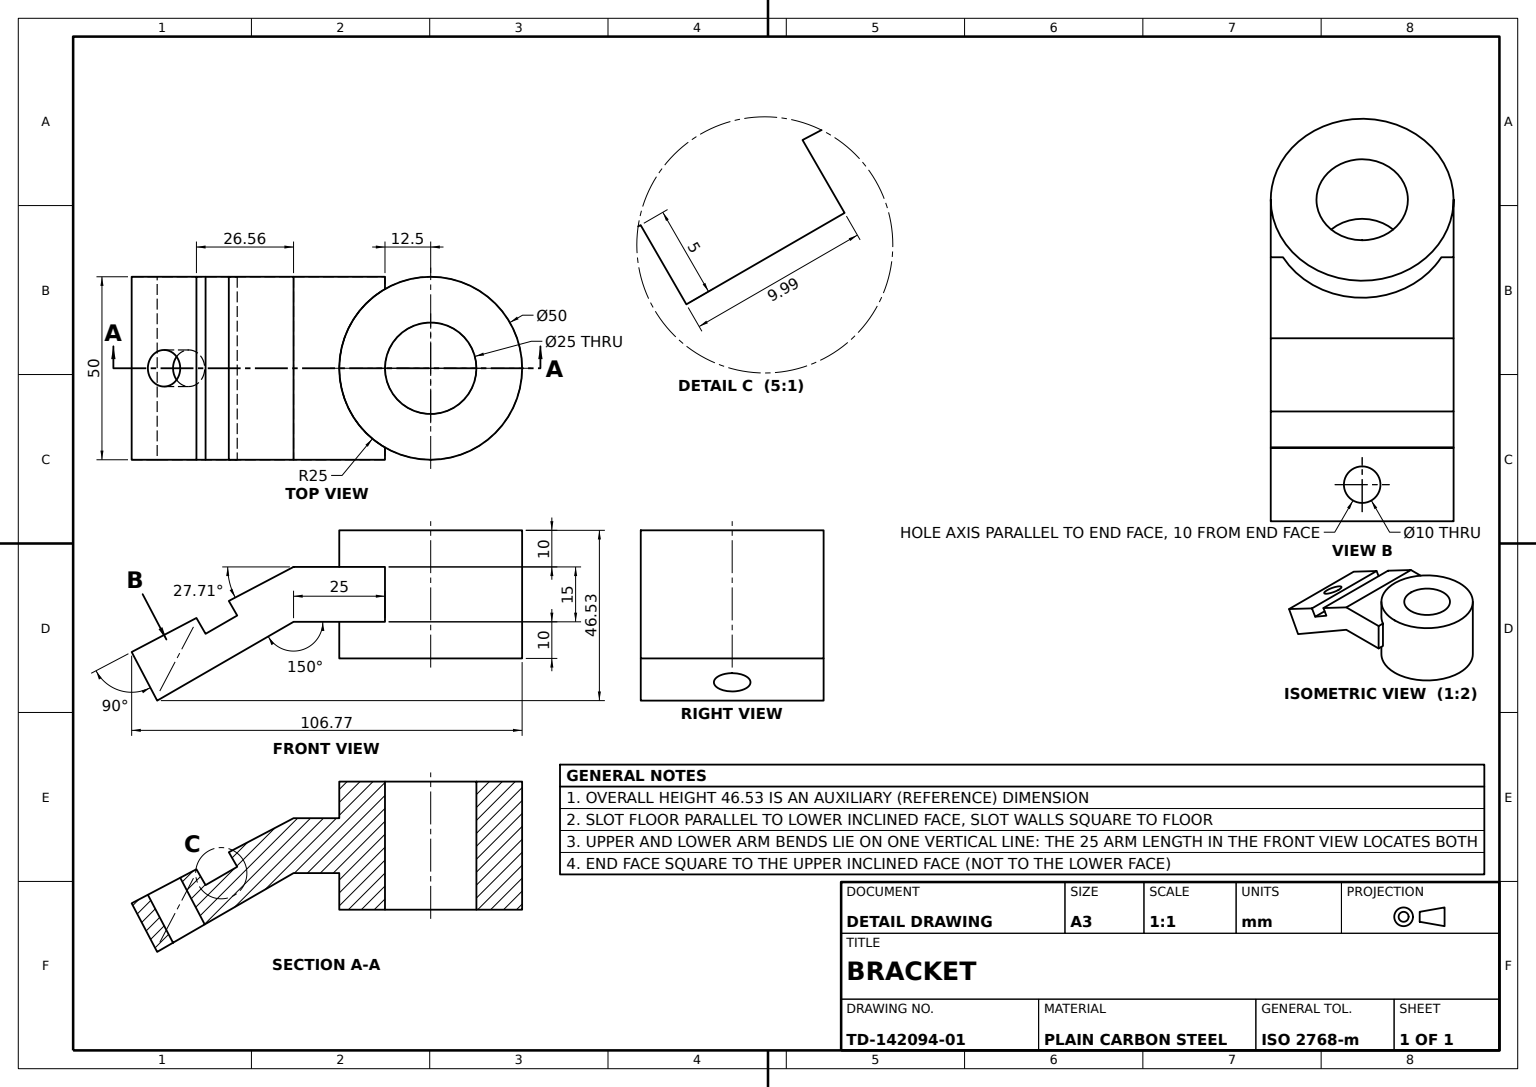
SolidWorks part; units mm, degrees
material "Plain Carbon Steel"
ref_plane "Front Plane" through (0, 0, 0) normal (0, 0, 1) x (1, 0, 0)
ref_plane "Top Plane" through (0, 0, 0) normal (0, 1, 0) x (1, 0, 0)
ref_plane "Right Plane" through (0, 0, 0) normal (1, 0, 0) x (0, 0, -1)
sketch "Base Profile Sketch" plane through (0, 0, 0) normal (0, 0, 1) x (1, 0, 0)
  line L0 (0, 0) -> (-25, 0)
  line L1 (-25, 0) -> (-62.2905, -21.5297)
  line L2 (-69.2655, -8.25) -> (-62.2905, -21.5297)
  line L3 (-69.2655, -8.25) -> (-25, 15)
  line L4 (-25, 15) -> (0, 15)
  line L5 (0, 0) -> (0, 15)
  dimension "D1" = 15
  dimension "D2" = 50
  dimension "D3" = 15
  dimension "D4" = 25
  dimension "D5" = 25
  dimension "D6" = 150
  dimension "D7" = 90
extrude "Base Block" add sketch "Base Profile Sketch" along normal mid plane 50
sketch "Cylinder Boss Sketch" plane through (0, 0, 0) normal (0, 1, 0) x (1, 0, 0)
  line L0 (0, 0) -> (12.5, 0)
  circle A0 centre (12.5, 0) radius 25
  dimension "D2" = 50
  dimension "D1" = 12.5
extrude "Cylinder Boss Ø50" add sketch "Cylinder Boss Sketch" along normal blind 25
sketch "Web Boss Sketch" plane through (0, 0, 0) normal (0, -1, 0) x (1, 0, 0)
  line L5 (0, -25) -> (0, -21.6506)
  line L6 (0, 21.6506) -> (0, 25)
  line L7 (0, 25) -> (-25, 25)
  line L8 (-25, 25) -> (-25, -25)
  line L9 (-25, -25) -> (0, -25)
  line L10 (0, -25) -> (0, -21.6506)
  line L11 (0, 21.6506) -> (0, 25)
  line L12 (0, 25) -> (-25, 25)
  line L13 (-25, 25) -> (-25, -25)
  line L14 (-25, -25) -> (0, -25)
  circle A0 centre (12.5, 0) radius 25
  arc A1 (0, -21.6506) -> (0, 21.6506) centre (12.5, 0) ccw
  arc A2 (0, -21.6506) -> (0, 21.6506) centre (12.5, 0) ccw
  arc M8 (0, -21.6506) -> (0, 21.6506) centre (12.5, 0) ccw
  dimension "D1" = 0
extrude "Web Boss" add sketch "Web Boss Sketch" along normal blind 10 contours A0 M8
sketch "Bore Sketch" plane through (0, -10, 0) normal (0, -1, 0) x (1, 0, 0)
  circle A0 centre (12.5, 0) radius 12.5
  circle A1 centre (12.5, 0) radius 25
  circle A2 centre (12.5, 0) radius 25
  dimension "D2" = 25
  dimension "D1" = 0
extrude "Bore Ø25" cut sketch "Bore Sketch" against normal through all contours A0
sketch "T-Slot Sketch" plane through (0, 0, 25) normal (0, 0, 1) x (1, 0, 0)
  line L0 (-47.1328, 3.375) -> (-40.1382, -8.74) construction
  line L1 (-51.4629, 0.875) -> (-44.4683, -11.24)
  line L2 (-42.7027, 5.7018) -> (-35.808, -6.24)
  line L3 (-51.4629, 0.875) -> (-48.9629, -3.4551)
  line L4 (-51.4629, 0.875) -> (-51.5558, 1.0518)
  line L5 (-51.5558, 1.0518) -> (-42.7027, 5.7018)
  line L6 (0, 0) -> (0, 15)
  line L7 (0, 15) -> (-25, 15)
  line L8 (-25, 15) -> (-69.2655, -8.25)
  line L9 (-69.2655, -8.25) -> (-62.2905, -21.5297)
  line L10 (-62.2905, -21.5297) -> (-25, 0)
  line L11 (-25, 0) -> (0, 0)
  line L12 (0, 0) -> (0, 15)
  line L13 (0, 15) -> (-25, 15)
  line L14 (-25, 15) -> (-69.2655, -8.25)
  line L16 (-62.2905, -21.5297) -> (-25, 0)
  line L17 (-25, 0) -> (0, 0)
  line L18 (-42.8026, 5.875) -> (-35.808, -6.24) construction
  line L19 (-51.5558, 1.0518) -> (-49.0558, -3.2783)
  line L20 (-49.0558, -3.2783) -> (-40.4024, 1.7177)
  line L21 (-51.5558, 1.0518) -> (-42.7027, 5.7018)
  line M11 (-25, 15) -> (-69.2655, -8.25)
  dimension "D4" = 5
  dimension "D1" = 0
  dimension "D2" = 5
  dimension "D3" = 5
extrude "T-Slot Cut" cut sketch "T-Slot Sketch" against normal through all contours L19 L20 L2 M11
sketch "Hole Sketch" plane through (-11.5807, 22.0484, 0) normal (-0.465, 0.8853, 0) x (0.8853, 0.465, 0)
  line L0 (-65.1578, 0) -> (-45.1538, 0) construction
  line L1 (-65.1578, -25) -> (-65.1578, 25) construction
  line L2 (-45.1538, 25) -> (-45.1538, -25) construction
  circle A0 centre (-55.1558, 0) radius 5
  dimension "D1" = 10
extrude "Hole Ø10" cut sketch "Hole Sketch" against normal through all
